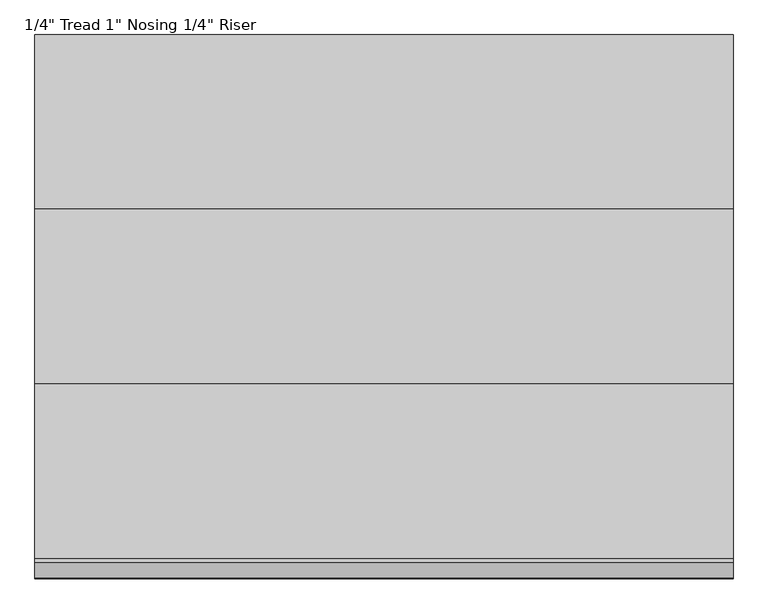
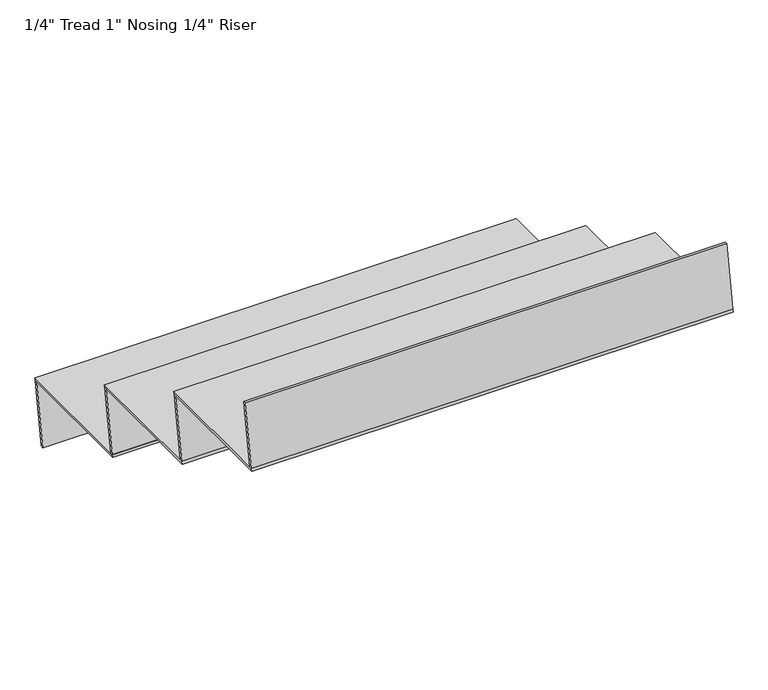
"""IFC4 building model written with IfcOpenShell, lengths in millimetres: stair flight geometry."""

from ifc_helpers import new_model, si_unit, frame, origin, place, context, project, spatial, polyline, outline, extrude, source, transform, mapped, element, save


def stair_flight_307daca0(model_context):
    return source(origin(), model_context, "Body", "SweptSolid", [
        extrude(outline(polyline([(5975.7902475, 152.4), (6287.0278379, 152.4), (6285.9695045, 146.05), (5974.7319142, 146.05), (5975.7902475, 152.4)])), frame((4466.3120815, 0.0, 0.0), z_axis=(1.0, 0.0, 0.0), x_axis=(0.0, 1.0, 0.0)), (0.0, 0.0, 1.0), 1117.6),
        extrude(outline(polyline([(6285.9695045, 146.05), (6261.6278379, 0.0), (6255.1902475, 0.0), (6279.5319142, 146.05), (6285.9695045, 146.05)])), frame((4466.3120815, 0.0, 0.0), z_axis=(1.0, 0.0, 0.0), x_axis=(0.0, 1.0, 0.0)), (0.0, 0.0, 1.0), 1117.6),
        extrude(outline(polyline([(6006.5695045, 298.45), (5982.2278379, 152.4), (5975.7902475, 152.4), (6000.1319142, 298.45), (6006.5695045, 298.45)])), frame((4466.3120815, 0.0, 0.0), z_axis=(1.0, 0.0, 0.0), x_axis=(0.0, 1.0, 0.0)), (0.0, 0.0, 1.0), 1117.6),
        extrude(outline(polyline([(5696.3902475, 304.8), (6007.6278379, 304.8), (6006.5695045, 298.45), (5695.3319142, 298.45), (5696.3902475, 304.8)])), frame((4466.3120815, 0.0, 0.0), z_axis=(1.0, 0.0, 0.0), x_axis=(0.0, 1.0, 0.0)), (0.0, 0.0, 1.0), 1117.6),
        extrude(outline(polyline([(5727.1695045, 450.85), (5702.8278379, 304.8), (5696.3902475, 304.8), (5720.7319142, 450.85), (5727.1695045, 450.85)])), frame((4466.3120815, 0.0, 0.0), z_axis=(1.0, 0.0, 0.0), x_axis=(0.0, 1.0, 0.0)), (0.0, 0.0, 1.0), 1117.6),
        extrude(outline(polyline([(5447.7695045, 603.25), (5423.4278379, 457.2), (5416.9902475, 457.2), (5441.3319142, 603.25), (5447.7695045, 603.25)])), frame((4466.3120815, 0.0, 0.0), z_axis=(1.0, 0.0, 0.0), x_axis=(0.0, 1.0, 0.0)), (0.0, 0.0, 1.0), 1117.6),
        extrude(outline(polyline([(5416.9902475, 457.2), (5728.2278379, 457.2), (5727.1695045, 450.85), (5415.9319142, 450.85), (5416.9902475, 457.2)])), frame((4466.3120815, 0.0, 0.0), z_axis=(1.0, 0.0, 0.0), x_axis=(0.0, 1.0, 0.0)), (0.0, 0.0, 1.0), 1117.6),
    ])


if __name__ == "__main__":
    model = new_model("IFC4")
    model_context = context("Model", 3, world=origin())
    ifc_project = project(units=[si_unit("LENGTHUNIT", "METRE", prefix="MILLI")], contexts=[model_context])
    site = spatial("IfcSite", under=ifc_project)
    building = spatial("IfcBuilding", under=site)
    placement = place(None, origin())
    stair_flight_shape = stair_flight_307daca0(model_context)
    element("IfcStairFlight", 1, ObjectType="1/4\" Tread 1\" Nosing 1/4\" Riser", at=placement, inside=building, context=model_context, shape_type="MappedRepresentation", body=[
        mapped(stair_flight_shape, transform((0.0, 0.0, 0.0), x_axis=(1.0, 0.0, 0.0), y_axis=(0.0, 1.0, 0.0), z_axis=(0.0, 0.0, 1.0))),
    ])
    save(model, "model.ifc")

# Revit data of these elements
# Element 1 (IfcStairFlight, "1/4\" Tread 1\" Nosing 1/4\" Riser")
#   Materials on its faces: "Steel, Paint Finish, Dark Gray"
# Materials
#   "Steel, Paint Finish, Dark Gray": class "Metal", colour RGB 89 89 89, transparency 0, Description = "Steel, paint finish, dark gray, glossy", Cost = 0
